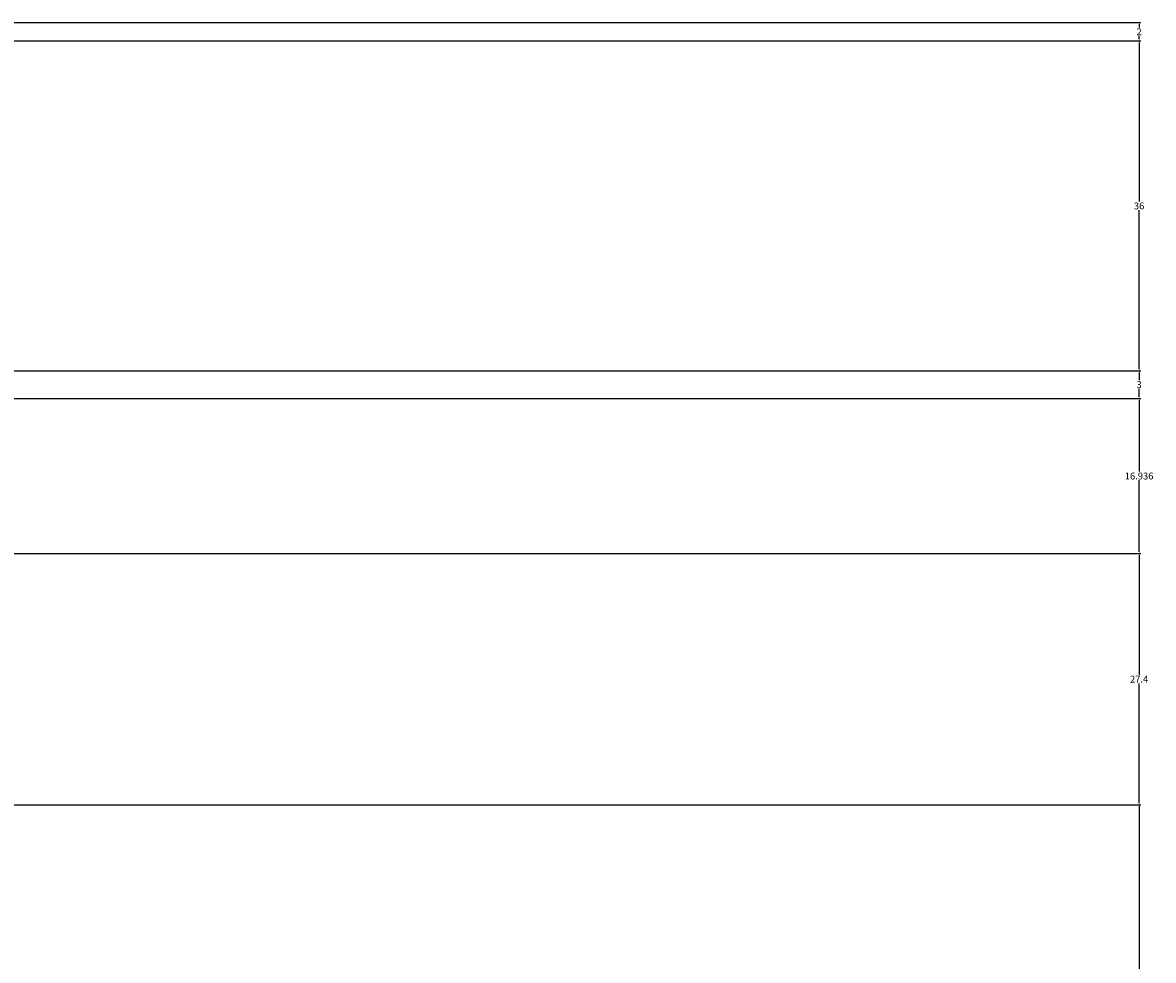
# Model space of a CAD drawing. Units: inches. Extents: x 62 to 566, y 66 to 528.
# Tile 20 of 20: x 443 to 566, y 401 to 503. Entities that reach past the tile are written whole.
import ezdxf

# ---------------------------------------------------------------- set-up
doc = ezdxf.new("R2010")
doc.units = ezdxf.units.IN
doc.header["$MEASUREMENT"] = 0
doc.layers.add('A-ANNO-DIMS', color=2, linetype='Continuous', lineweight=18)
doc.styles.get("Standard").update_dxf_attribs({"font": 'arial.ttf'})
doc.dimstyles.get("Standard").update_dxf_attribs({"dimtxt": 0.75, "dimasz": 0.18, "dimexe": 0.18, "dimexo": 0.0625, "dimgap": 0.09, "dimtad": 0, "dimtih": 1, "dimtoh": 1, "dimdec": 4, "dimzin": 0, "dimdsep": 46, "dimlunit": 4, "dimtxsty": 'Standard', "dimcen": 0.09, "dimadec": 0, "dimazin": 0, "dimtfac": 1, "dimtdec": 4, "dimtofl": 0, "dimtmove": 0, "dimatfit": 3, "dimfxl": 1, "dimtolj": 1, "dimtzin": 0, "dimarcsym": 0})

# ---------------------------------------------------------------- blocks, each defined once
blk = doc.blocks.new('*D24')
at = {"layer": 'A-ANNO-DIMS', "color": 0, "lineweight": -2, "transparency": 16777216}
for p, q in [((374.2, 417.71), (564.47, 417.71)), ((564.29, 417.53), (564.29, 381.72)), ((564.29, 344.96), (564.29, 380.77)), ((374.2, 344.78), (564.47, 344.78))]:
    blk.add_line(p, q, dxfattribs=at)
at = {"layer": 'A-ANNO-DIMS', "color": 0, "transparency": 16777216}
for points in [[(564.26, 417.53), (564.32, 417.53), (564.29, 417.71)], [(564.26, 344.96), (564.32, 344.96), (564.29, 344.78)]]:
    blk.add_solid(points, dxfattribs=at)
at = {"layer": 'Defpoints', "color": 0, "transparency": 16777216}
for p in [(374.14, 417.71), (564.29, 417.71), (374.14, 344.78)]:
    blk.add_point(p, dxfattribs=at)
at = {"layer": 'A-ANNO-DIMS', "color": 0, "transparency": 16777216, "insert": (564.29, 381.24), "char_height": 0.75, "attachment_point": 5}
blk.add_mtext('\\A1;72.92', dxfattribs=at)
blk = doc.blocks.new('*D52')
at = {"layer": 'A-ANNO-DIMS', "color": 0, "lineweight": -2, "transparency": 16777216}
for p, q in [((430.76, 445.11), (564.47, 445.11)), ((564.29, 444.93), (564.29, 431.87)), ((564.29, 417.89), (564.29, 430.94)), ((374.2, 417.71), (564.47, 417.71))]:
    blk.add_line(p, q, dxfattribs=at)
at = {"layer": 'A-ANNO-DIMS', "color": 0, "transparency": 16777216}
for points in [[(564.26, 444.93), (564.32, 444.93), (564.29, 445.11)], [(564.26, 417.89), (564.32, 417.89), (564.29, 417.71)]]:
    blk.add_solid(points, dxfattribs=at)
at = {"layer": 'Defpoints', "color": 0, "transparency": 16777216}
for p in [(430.69, 445.11), (564.29, 445.11), (374.14, 417.71)]:
    blk.add_point(p, dxfattribs=at)
at = {"layer": 'A-ANNO-DIMS', "color": 0, "transparency": 16777216, "insert": (564.29, 431.41), "char_height": 0.75, "attachment_point": 5}
blk.add_mtext('\\A1;27.4', dxfattribs=at)
blk = doc.blocks.new('*D53')
at = {"layer": 'A-ANNO-DIMS', "color": 0, "lineweight": -2, "transparency": 16777216}
for p, q in [((430.76, 462.04), (564.47, 462.04)), ((564.29, 461.86), (564.29, 454.05)), ((564.29, 445.29), (564.29, 453.1)), ((430.76, 445.11), (564.47, 445.11))]:
    blk.add_line(p, q, dxfattribs=at)
at = {"layer": 'A-ANNO-DIMS', "color": 0, "transparency": 16777216}
for points in [[(564.26, 461.86), (564.32, 461.86), (564.29, 462.04)], [(564.26, 445.29), (564.32, 445.29), (564.29, 445.11)]]:
    blk.add_solid(points, dxfattribs=at)
at = {"layer": 'Defpoints', "color": 0, "transparency": 16777216}
for p in [(430.69, 462.04), (564.29, 462.04), (430.69, 445.11)]:
    blk.add_point(p, dxfattribs=at)
at = {"layer": 'A-ANNO-DIMS', "color": 0, "transparency": 16777216, "insert": (564.29, 453.57), "char_height": 0.75, "attachment_point": 5}
blk.add_mtext('\\A1;16.936', dxfattribs=at)
blk = doc.blocks.new('*D54')
at = {"layer": 'A-ANNO-DIMS', "color": 0, "lineweight": -2, "transparency": 16777216}
for p, q in [((430.76, 465.04), (564.47, 465.04)), ((564.29, 464.86), (564.29, 464.02)), ((564.29, 462.22), (564.29, 463.07)), ((430.76, 462.04), (564.47, 462.04))]:
    blk.add_line(p, q, dxfattribs=at)
at = {"layer": 'A-ANNO-DIMS', "color": 0, "transparency": 16777216}
for points in [[(564.26, 464.86), (564.32, 464.86), (564.29, 465.04)], [(564.26, 462.22), (564.32, 462.22), (564.29, 462.04)]]:
    blk.add_solid(points, dxfattribs=at)
at = {"layer": 'Defpoints', "color": 0, "transparency": 16777216}
for p in [(430.69, 465.04), (564.29, 465.04), (430.69, 462.04)]:
    blk.add_point(p, dxfattribs=at)
at = {"layer": 'A-ANNO-DIMS', "color": 0, "transparency": 16777216, "insert": (564.29, 463.54), "char_height": 0.75, "attachment_point": 5}
blk.add_mtext('\\A1;3', dxfattribs=at)
blk = doc.blocks.new('*D55')
at = {"layer": 'A-ANNO-DIMS', "color": 0, "lineweight": -2, "transparency": 16777216}
for p, q in [((430.76, 501.04), (564.47, 501.04)), ((564.29, 500.86), (564.29, 483.52)), ((564.29, 465.22), (564.29, 482.57)), ((430.76, 465.04), (564.47, 465.04))]:
    blk.add_line(p, q, dxfattribs=at)
at = {"layer": 'A-ANNO-DIMS', "color": 0, "transparency": 16777216}
for points in [[(564.26, 500.86), (564.32, 500.86), (564.29, 501.04)], [(564.26, 465.22), (564.32, 465.22), (564.29, 465.04)]]:
    blk.add_solid(points, dxfattribs=at)
at = {"layer": 'Defpoints', "color": 0, "transparency": 16777216}
for p in [(430.69, 501.04), (564.29, 501.04), (430.69, 465.04)]:
    blk.add_point(p, dxfattribs=at)
at = {"layer": 'A-ANNO-DIMS', "color": 0, "transparency": 16777216, "insert": (564.29, 483.04), "char_height": 0.75, "attachment_point": 5}
blk.add_mtext('\\A1;36', dxfattribs=at)
blk = doc.blocks.new('*D56')
at = {"layer": 'A-ANNO-DIMS', "color": 0, "lineweight": -2, "transparency": 16777216}
for p, q in [((435.46, 503.04), (564.47, 503.04)), ((564.29, 502.86), (564.29, 502.51)), ((430.76, 501.04), (564.47, 501.04)), ((564.29, 501.22), (564.29, 501.58))]:
    blk.add_line(p, q, dxfattribs=at)
at = {"layer": 'A-ANNO-DIMS', "color": 0, "transparency": 16777216}
for points in [[(564.26, 502.86), (564.32, 502.86), (564.29, 503.04)], [(564.26, 501.22), (564.32, 501.22), (564.29, 501.04)]]:
    blk.add_solid(points, dxfattribs=at)
at = {"layer": 'Defpoints', "color": 0, "transparency": 16777216}
for p in [(435.39, 503.04), (564.29, 503.04), (430.69, 501.04)]:
    blk.add_point(p, dxfattribs=at)
at = {"layer": 'A-ANNO-DIMS', "color": 0, "transparency": 16777216, "insert": (564.29, 502.04), "char_height": 0.75, "attachment_point": 5}
blk.add_mtext('\\A1;2', dxfattribs=at)

msp = doc.modelspace()

# ---------------------------------------------------------------- dimensions: what is measured, and where the dimension line sits
at = {"layer": 'A-ANNO-DIMS'}
for base, p1, p2, override, picture, middle in [((564.2868, 503.0423), (430.6938, 501.0423), (435.3945, 503.0423), {"dimdec": 0, "dimlfac": 1, "dimrnd": 0, "dimzin": 0, "dimdsep": 46, "dimlunit": 2}, '*D56', (564.2868, 502.0423)), ((564.2868, 501.0423), (430.6938, 465.0423), (430.6938, 501.0423), {"dimdec": 0, "dimlfac": 1, "dimrnd": 0, "dimzin": 0, "dimdsep": 46, "dimlunit": 2}, '*D55', (564.2868, 483.0423)), ((564.2868, 465.0423), (430.6938, 462.0423), (430.6938, 465.0423), {"dimdec": 0, "dimlfac": 1, "dimrnd": 0, "dimzin": 0, "dimdsep": 46, "dimlunit": 2}, '*D54', (564.2868, 463.5423)), ((564.2868, 462.0423), (430.6938, 445.1064), (430.6938, 462.0423), {"dimdec": 3, "dimlfac": 1, "dimrnd": 0, "dimzin": 0, "dimdsep": 46, "dimlunit": 2}, '*D53', (564.2868, 453.5744)), ((564.2868, 445.1064), (374.1373, 417.7059), (430.6938, 445.1064), {"dimdec": 1, "dimlfac": 1, "dimrnd": 0, "dimzin": 0, "dimdsep": 46, "dimlunit": 2}, '*D52', (564.2868, 431.4062)), ((564.2868, 417.7059), (374.1373, 344.7821), (374.1373, 417.7059), {"dimdec": 2, "dimlfac": 1, "dimrnd": 0, "dimzin": 0, "dimdsep": 46, "dimlunit": 2}, '*D24', (564.2868, 381.244))]:
    dim = msp.add_linear_dim(base=base, p1=p1, p2=p2, angle=90, dimstyle='Standard', override=override, dxfattribs=at)
    dim.commit()
    dim.dimension.update_dxf_attribs({"geometry": picture, "text_midpoint": middle})

doc.saveas('drawing.dxf')
